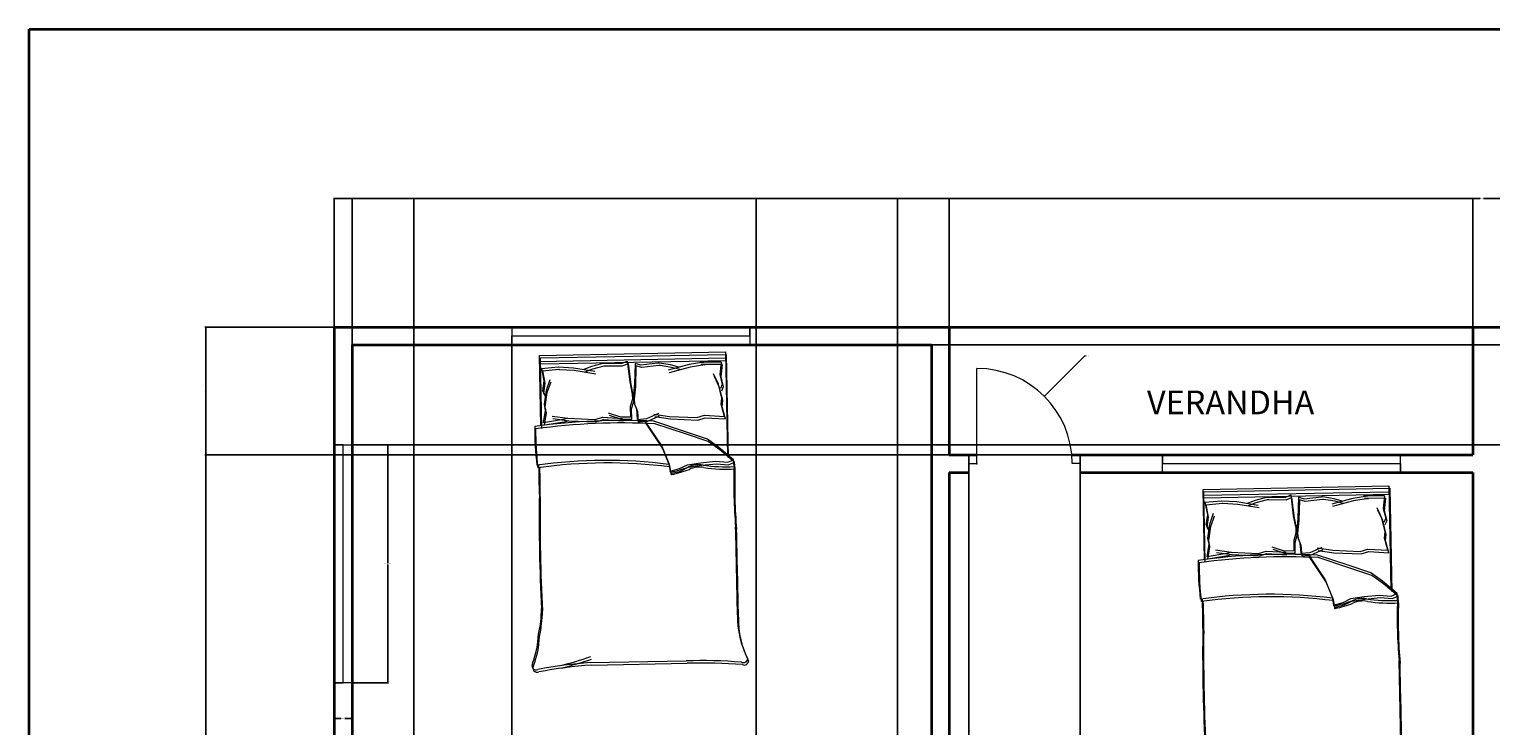
# Model space of a CAD drawing. Units: inches. Extents: x 1721 to 2510, y 1544 to 2360.
# Tile 8 of 10: x 1721 to 2090, y 2185 to 2360. Entities that reach past the tile are written whole.
import ezdxf

# ---------------------------------------------------------------- set-up
doc = ezdxf.new("R2010")
doc.units = ezdxf.units.IN
for name, color, linetype, lineweight in [('A-ANNO-DIMS', 2, 'Continuous', 18), ('A-ANNO-TTLB', 7, 'Continuous', 35), ('A-AREA-IDEN', 7, 'Continuous', 18), ('A-DOOR', 3, 'Continuous', 18), ('A-FURN', 8, 'Continuous', 13), ('A-GLAZ', 4, 'Continuous', 18), ('A-WALL', 7, 'Continuous', 35)]:
    doc.layers.add(name, color=color, linetype=linetype, lineweight=lineweight)
doc.styles.get("Standard").update_dxf_attribs({"font": 'arial.ttf'})
doc.dimstyles.get("Standard").update_dxf_attribs({"dimtxt": 0.18, "dimasz": 0.18, "dimexe": 0.18, "dimexo": 0.0625, "dimgap": 0.09, "dimtad": 0, "dimtih": 1, "dimtoh": 1, "dimdec": 4, "dimzin": 0, "dimdsep": 46, "dimtxsty": 'Standard', "dimcen": 0.09, "dimadec": 0, "dimazin": 0, "dimtfac": 1, "dimtdec": 4, "dimtofl": 0, "dimtmove": 0, "dimatfit": 3, "dimfxl": 1, "dimtolj": 1, "dimtzin": 0, "dimarcsym": 0})

# ---------------------------------------------------------------- blocks, each defined once
blk = doc.blocks.new('BED-DOUBLE')
for p, q in [((39.64, 78.43), (15.52, 78.72)), ((39.64, 78.43), (15.52, 78.72)), ((39.86, 77.8), (15.74, 78.09)), ((39.86, 77.8), (15.74, 78.09)), ((1.93, 30.11), (1.99, 28.4, 3.79)), ((1.93, 30.11), (1.99, 28.4, 3.79)), ((2.15, 29.48), (2.21, 27.77, 3.79)), ((2.15, 29.48), (2.21, 27.77, 3.79)), ((15.66, 30.21), (13.68, 29.32)), ((15.66, 30.21), (13.68, 29.32)), ((15.88, 29.58), (13.89, 28.69)), ((15.88, 29.58), (13.89, 28.69)), ((18.1, 30.79), (15.66, 30.21)), ((18.1, 30.79), (15.66, 30.21)), ((18.31, 30.16), (15.88, 29.58)), ((18.31, 30.16), (15.88, 29.58)), ((18.38, 28.81), (18.1, 30.79)), ((18.38, 28.81), (18.1, 30.79)), ((18.59, 28.18), (18.31, 30.16)), ((18.59, 28.18), (18.31, 30.16)), ((3.5, 28.99), (1.99, 28.4)), ((3.5, 28.99), (1.99, 28.4)), ((1.99, 28.4), (5.58, 25.17)), ((1.99, 28.4), (5.58, 25.17)), ((3.72, 28.36), (2.21, 27.77)), ((3.72, 28.36), (2.21, 27.77)), ((2.21, 27.77), (5.8, 24.54)), ((2.21, 27.77), (5.8, 24.54)), ((3.23, 1.19), (3.55, 27.27)), ((3.23, 1.19), (3.55, 27.27)), ((3.45, 0.56), (3.76, 26.64)), ((3.45, 0.56), (3.76, 26.64)), ((6.54, 28.65), (3.5, 28.99)), ((6.54, 28.65), (3.5, 28.99)), ((6.75, 28.02), (3.72, 28.36)), ((6.75, 28.02), (3.72, 28.36)), ((10.33, 28.91), (6.54, 28.65)), ((10.33, 28.91), (6.54, 28.65)), ((10.55, 28.28), (6.75, 28.02)), ((10.55, 28.28), (6.75, 28.02)), ((13.68, 29.32), (10.33, 28.91)), ((13.68, 29.32), (10.33, 28.91)), ((13.89, 28.69), (10.55, 28.28)), ((13.89, 28.69), (10.55, 28.28)), ((20, 24.39), (18.38, 28.81)), ((20, 24.39), (18.38, 28.81)), ((20.21, 23.76), (18.59, 28.18)), ((20.21, 23.76), (18.59, 28.18)), ((5.58, 25.17), (8.44, 23.01)), ((5.58, 25.17), (8.44, 23.01)), ((5.8, 24.54), (8.66, 22.38)), ((5.8, 24.54), (8.66, 22.38)), ((8.44, 23.01), (13.88, 20.98)), ((8.44, 23.01), (13.88, 20.98)), ((8.66, 22.38), (14.1, 20.35)), ((8.66, 22.38), (14.1, 20.35)), ((24.03, 17.98), (20, 24.39)), ((24.03, 17.98), (20, 24.39)), ((24.24, 17.35), (20.21, 23.76)), ((24.24, 17.35), (20.21, 23.76)), ((13.88, 20.98), (22.02, 18)), ((13.88, 20.98), (22.02, 18)), ((14.1, 20.35), (22.24, 17.37)), ((14.1, 20.35), (22.24, 17.37)), ((9.01, 16.97), (3.98, 17.42)), ((3.98, 17.42), (4.71, 14.34)), ((9.01, 16.97), (3.98, 17.42)), ((3.98, 17.42), (4.71, 14.34)), ((9.23, 16.34), (4.2, 16.8)), ((4.2, 16.8), (4.92, 13.71)), ((9.23, 16.34), (4.2, 16.8)), ((4.2, 16.8), (4.92, 13.71)), ((10.94, 17.49), (9.01, 16.97)), ((10.94, 17.49), (9.01, 16.97)), ((11.15, 16.86), (9.23, 16.34)), ((11.15, 16.86), (9.23, 16.34)), ((17.8, 16.99), (10.94, 17.49)), ((17.8, 16.99), (10.94, 17.49)), ((18.02, 16.36), (11.15, 16.86)), ((18.02, 16.36), (11.15, 16.86)), ((21.75, 16.29), (17.8, 16.99)), ((21.75, 16.29), (17.8, 16.99)), ((21.96, 15.66), (18.02, 16.36)), ((21.96, 15.66), (18.02, 16.36)), ((23.54, 17.35), (20.51, 16.13)), ((23.54, 17.35), (20.51, 16.13)), ((23.75, 16.73), (20.73, 15.5)), ((23.75, 16.73), (20.73, 15.5)), ((25.94, 17.48), (23.54, 17.35)), ((25.94, 17.48), (23.54, 17.35)), ((26.16, 16.85), (23.75, 16.73)), ((26.16, 16.85), (23.75, 16.73)), ((26.07, 14.85), (25.94, 17.48)), ((26.07, 14.85), (25.94, 17.48)), ((26.73, 13.04), (26.07, 14.85)), ((26.73, 13.04), (26.07, 14.85)), ((26.29, 14.22), (26.16, 16.85)), ((26.29, 14.22), (26.16, 16.85)), ((27.61, 14.21), (27.64, 16.84)), ((27.61, 14.21), (27.64, 16.84)), ((27.64, 16.84), (30.05, 16.81)), ((27.64, 16.84), (30.05, 16.81)), ((27.82, 13.58), (27.85, 16.21)), ((27.82, 13.58), (27.85, 16.21)), ((27.85, 16.21), (30.26, 16.18)), ((27.85, 16.21), (30.26, 16.18)), ((34.67, 16.66), (29.65, 17.12)), ((34.67, 16.66), (29.65, 17.12)), ((34.89, 16.03), (29.86, 16.49)), ((34.89, 16.03), (29.86, 16.49)), ((30.05, 16.81), (33.11, 15.7)), ((30.05, 16.81), (33.11, 15.7)), ((30.26, 16.18), (33.33, 15.07)), ((30.26, 16.18), (33.33, 15.07)), ((36.6, 17.19), (34.67, 16.66)), ((36.6, 17.19), (34.67, 16.66)), ((36.81, 16.56), (34.89, 16.03)), ((36.81, 16.56), (34.89, 16.03)), ((43.46, 16.68), (36.6, 17.19)), ((43.46, 16.68), (36.6, 17.19)), ((43.68, 16.05), (36.81, 16.56)), ((43.68, 16.05), (36.81, 16.56)), ((43.46, 16.68), (44.58, 16.98)), ((43.46, 16.68), (44.58, 16.98)), ((47.41, 15.98), (43.46, 16.68)), ((47.41, 15.98), (43.46, 16.68)), ((43.68, 16.05), (44.79, 16.35)), ((43.68, 16.05), (44.79, 16.35)), ((47.62, 15.35), (43.68, 16.05)), ((47.62, 15.35), (43.68, 16.05)), ((44.58, 16.98), (49.58, 17.63)), ((44.58, 16.98), (49.58, 17.63)), ((44.79, 16.35), (49.8, 17)), ((44.79, 16.35), (49.8, 17)), ((49.58, 17.63), (48.98, 14.52)), ((49.58, 17.63), (48.98, 14.52)), ((49.8, 17), (49.19, 13.89)), ((49.8, 17), (49.19, 13.89)), ((50.28, 18.38), (50.07, 0.63)), ((50.28, 18.38), (50.07, 0.63)), ((50.5, 17.75), (50.29, 0)), ((50.5, 17.75), (50.29, 0)), ((4.71, 14.34), (4.5, 12.77)), ((4.71, 14.34), (4.5, 12.77)), ((4.5, 12.77), (5.25, 9.26)), ((4.5, 12.77), (5.25, 9.26)), ((4.92, 13.71), (4.72, 12.14)), ((4.92, 13.71), (4.72, 12.14)), ((4.72, 12.14), (5.46, 8.63)), ((4.72, 12.14), (5.46, 8.63)), ((26.95, 12.41), (26.29, 14.22)), ((26.95, 12.41), (26.29, 14.22)), ((26.39, 8.62), (26.8, 11.77)), ((26.39, 8.62), (26.8, 11.77)), ((26.61, 7.99), (27.01, 11.14)), ((26.61, 7.99), (27.01, 11.14)), ((26.8, 11.77), (26.73, 13.04)), ((26.8, 11.77), (26.73, 13.04)), ((27.01, 11.14), (26.95, 12.41)), ((27.01, 11.14), (26.95, 12.41)), ((27, 11.1), (27.02, 12.38)), ((27, 11.1), (27.02, 12.38)), ((27.53, 7.98), (27, 11.1)), ((27.53, 7.98), (27, 11.1)), ((27.02, 12.38), (27.61, 14.21)), ((27.02, 12.38), (27.61, 14.21)), ((27.22, 10.47), (27.23, 11.75)), ((27.22, 10.47), (27.23, 11.75)), ((27.23, 11.75), (27.82, 13.58)), ((27.23, 11.75), (27.82, 13.58)), ((49.24, 12.96), (48.63, 9.42)), ((49.24, 12.96), (48.63, 9.42)), ((49.46, 12.33), (48.85, 8.79)), ((49.46, 12.33), (48.85, 8.79)), ((48.98, 14.52), (49.24, 12.96)), ((48.98, 14.52), (49.24, 12.96)), ((49.19, 13.89), (49.46, 12.33)), ((49.19, 13.89), (49.46, 12.33)), ((4.25, 9.35), (4.77, 10.37)), ((4.25, 9.35), (4.77, 10.37)), ((4.8, 6.82), (4.25, 9.35)), ((4.8, 6.82), (4.25, 9.35)), ((4.47, 8.72), (4.98, 9.74)), ((4.47, 8.72), (4.98, 9.74)), ((5.02, 6.19), (4.47, 8.72)), ((5.02, 6.19), (4.47, 8.72)), ((5.25, 9.26), (6.37, 6.62)), ((5.25, 9.26), (6.37, 6.62)), ((5.46, 8.63), (6.59, 5.99)), ((5.46, 8.63), (6.59, 5.99)), ((26.09, 3.36), (26.39, 8.62)), ((26.09, 3.36), (26.39, 8.62)), ((26.3, 2.73), (26.61, 7.99)), ((26.3, 2.73), (26.61, 7.99)), ((27.75, 7.35), (27.22, 10.47)), ((27.75, 7.35), (27.22, 10.47)), ((28.04, 2.73), (27.53, 7.98)), ((28.04, 2.73), (27.53, 7.98)), ((48.63, 9.42), (47.61, 6.74)), ((48.63, 9.42), (47.61, 6.74)), ((48.85, 8.79), (47.82, 6.11)), ((48.85, 8.79), (47.82, 6.11)), ((49.63, 9.55), (49.07, 10.55)), ((49.63, 9.55), (49.07, 10.55)), ((49.17, 7.01), (49.63, 9.55)), ((49.17, 7.01), (49.63, 9.55)), ((49.84, 8.92), (49.29, 9.92)), ((49.84, 8.92), (49.29, 9.92)), ((49.39, 6.38), (49.84, 8.92)), ((49.39, 6.38), (49.84, 8.92)), ((4.39, 3.68), (4.8, 6.82)), ((4.39, 3.68), (4.8, 6.82)), ((4.61, 3.05), (5.02, 6.19)), ((4.61, 3.05), (5.02, 6.19)), ((8.71, 3.62), (12.44, 4.09)), ((8.71, 3.62), (12.44, 4.09)), ((12.44, 4.09), (17.76, 5.35)), ((12.44, 4.09), (17.76, 5.35)), ((12.65, 3.46), (17.98, 4.72)), ((12.65, 3.46), (17.98, 4.72)), ((15.1, 4.65), (17.12, 4.04)), ((15.1, 4.65), (17.12, 4.04)), ((15.32, 4.02), (17.34, 3.41)), ((15.32, 4.02), (17.34, 3.41)), ((17.12, 4.04), (19.98, 3.48)), ((17.12, 4.04), (19.98, 3.48)), ((20.3, 3.49), (24.64, 3.85)), ((20.3, 3.49), (24.64, 3.85)), ((24.64, 3.85), (26.09, 3.36)), ((24.64, 3.85), (26.09, 3.36)), ((28.25, 2.1), (27.75, 7.35)), ((28.25, 2.1), (27.75, 7.35)), ((36.97, 3.75), (34.13, 3.08)), ((36.97, 3.75), (34.13, 3.08)), ((41.65, 3.98), (36.28, 5.04)), ((41.65, 3.98), (36.28, 5.04)), ((41.87, 3.35), (36.49, 4.41)), ((41.87, 3.35), (36.49, 4.41)), ((38.96, 4.44), (36.97, 3.75)), ((38.96, 4.44), (36.97, 3.75)), ((39.18, 3.81), (37.19, 3.12)), ((39.18, 3.81), (37.19, 3.12)), ((45.39, 3.65), (41.65, 3.98)), ((45.39, 3.65), (41.65, 3.98)), ((49.7, 3.91), (45.5, 3.63)), ((49.7, 3.91), (45.5, 3.63)), ((49.7, 3.88), (49.17, 7.01)), ((49.7, 3.88), (49.17, 7.01)), ((49.92, 3.25), (49.39, 6.38)), ((49.92, 3.25), (49.39, 6.38)), ((50.07, 0.63), (3.23, 1.19)), ((50.07, 0.63), (3.23, 1.19)), ((50.09, 2.13), (3.25, 2.69)), ((50.09, 2.13), (3.25, 2.69)), ((50.29, 0), (3.45, 0.56)), ((50.29, 0), (3.45, 0.56)), ((50.31, 1.5), (3.47, 2.06)), ((50.31, 1.5), (3.47, 2.06)), ((4.39, 3.68), (9.69, 3.52)), ((4.39, 3.68), (9.69, 3.52)), ((4.61, 3.05), (9.9, 2.89)), ((4.61, 3.05), (9.9, 2.89)), ((9.69, 3.52), (8.71, 3.62)), ((9.69, 3.52), (8.71, 3.62)), ((8.92, 2.99), (12.65, 3.46)), ((8.92, 2.99), (12.65, 3.46)), ((9.9, 2.89), (8.92, 2.99)), ((9.9, 2.89), (8.92, 2.99)), ((17.34, 3.41), (20.2, 2.85)), ((17.34, 3.41), (20.2, 2.85)), ((19.98, 3.48), (20.3, 3.49)), ((19.98, 3.48), (20.3, 3.49)), ((20.2, 2.85), (20.52, 2.86)), ((20.2, 2.85), (20.52, 2.86)), ((20.52, 2.86), (24.86, 3.22)), ((20.52, 2.86), (24.86, 3.22)), ((24.86, 3.22), (26.3, 2.73)), ((24.86, 3.22), (26.3, 2.73)), ((29.46, 3.28), (28.04, 2.73)), ((29.46, 3.28), (28.04, 2.73)), ((29.68, 2.65), (28.25, 2.1)), ((29.68, 2.65), (28.25, 2.1)), ((33.81, 3.08), (29.46, 3.28)), ((33.81, 3.08), (29.46, 3.28)), ((34.03, 2.45), (29.68, 2.65)), ((34.03, 2.45), (29.68, 2.65)), ((34.13, 3.08), (33.81, 3.08)), ((34.13, 3.08), (33.81, 3.08)), ((34.35, 2.45), (34.03, 2.45)), ((34.35, 2.45), (34.03, 2.45)), ((37.19, 3.12), (34.35, 2.45)), ((37.19, 3.12), (34.35, 2.45)), ((45.61, 3.02), (41.87, 3.35)), ((45.61, 3.02), (41.87, 3.35)), ((45.5, 3.63), (45.39, 3.65)), ((45.5, 3.63), (45.39, 3.65)), ((45.71, 3), (45.61, 3.02)), ((45.71, 3), (45.61, 3.02)), ((49.91, 3.28), (45.71, 3)), ((49.91, 3.28), (45.71, 3))]:
    blk.add_line(p, q)
for centre, radius, start, end in [((1.08, 78.52), 1.08, 61.9736, 175.3348), ((1.08, 78.52), 1.08, 61.9736, 175.3348), ((-20.36, 68.78), 22.61, 356.7862, 25.7829), ((-20.36, 68.78), 22.61, 356.7862, 25.7829), ((1.29, 77.89), 1.08, 61.9736, 175.3348), ((1.29, 77.89), 1.08, 61.9736, 175.3348), ((-20.14, 68.15), 22.61, 356.7862, 25.7829), ((-20.14, 68.15), 22.61, 356.7862, 25.7829), ((15.63, 209.12), 130.4, 263.8146, 269.9499), ((15.63, 209.12), 130.4, 263.8146, 269.9499), ((15.85, 208.49), 130.4, 263.8146, 269.9499), ((15.85, 208.49), 130.4, 263.8146, 269.9499), ((70.08, -22.85), 104.34, 102.698, 107.0202), ((70.08, -22.85), 104.34, 102.698, 107.0202), ((34.83, 197.67), 119.34, 272.3106, 278.7239), ((34.83, 197.67), 119.34, 272.3106, 278.7239), ((70.29, -23.48), 104.34, 102.698, 107.0202), ((70.29, -23.48), 104.34, 102.698, 107.0202), ((35.05, 197.04), 119.34, 272.3106, 278.7239), ((35.05, 197.04), 119.34, 272.3106, 278.7239), ((75.53, 69.21), 23.09, 157.2899, 175.9668), ((75.53, 69.21), 23.09, 157.2899, 175.9668), ((75.75, 68.58), 23.09, 157.2899, 175.9668), ((75.75, 68.58), 23.09, 157.2899, 175.9668), ((53.35, 78.73), 1.07, 325.4884, 112.793), ((53.35, 78.73), 1.07, 325.4884, 112.793), ((53.56, 78.1), 1.07, 325.4884, 112.793), ((53.56, 78.1), 1.07, 325.4884, 112.793), ((80.6, 63.5), 29.05, 165.3797, 178.2261), ((80.6, 63.5), 29.05, 165.3797, 178.2261), ((80.81, 62.87), 29.05, 165.3797, 178.2261), ((80.81, 62.87), 29.05, 165.3797, 178.2261), ((4473.12, 14.21), 4471.22, 179.317, 179.60172), ((4473.12, 14.21), 4471.22, 179.317, 179.60172), ((4473.34, 13.58), 4471.22, 179.317, 179.60172), ((4473.34, 13.58), 4471.22, 179.317, 179.60172), ((-421.08, 55.88), 472.73, 357.5425, 1.0334), ((-421.08, 55.88), 472.73, 357.5425, 1.0334), ((-420.87, 55.25), 472.73, 357.5425, 1.0334), ((-420.87, 55.25), 472.73, 357.5425, 1.0334), ((-124.73, 38.32), 126.93, 356.294, 3.1513), ((-124.73, 38.32), 126.93, 356.294, 3.1513), ((-124.51, 37.69), 126.93, 356.294, 3.1513), ((-124.51, 37.69), 126.93, 356.294, 3.1513), ((217.81, 29.18), 166.73, 177.791, 180.323), ((217.81, 29.18), 166.73, 177.791, 180.323), ((218.03, 28.55), 166.73, 177.791, 180.323), ((218.03, 28.55), 166.73, 177.791, 180.323), ((3.1, -5.33), 35.46, 79.1911, 91.8805), ((3.1, -5.33), 35.46, 79.1911, 91.8805), ((3.31, -5.96), 35.46, 79.1911, 91.8805), ((3.31, -5.96), 35.46, 79.1911, 91.8805), ((11.02, 35.47), 6.1, 257.9756, 293.0532), ((11.02, 35.47), 6.1, 257.9756, 293.0532), ((22.96, 2.41), 29.06, 99.9765, 109.1954), ((22.96, 2.41), 29.06, 99.9765, 109.1954), ((23.18, 1.78), 29.06, 99.9765, 109.1954), ((23.18, 1.78), 29.06, 99.9765, 109.1954), ((17.93, 30.85), 0.181, 339.5612, 90.4525), ((17.93, 30.85), 0.181, 339.5612, 90.4525), ((18.15, 30.22), 0.181, 339.5612, 90.4525), ((18.15, 30.22), 0.181, 339.5612, 90.4525), ((11.23, 34.84), 6.1, 257.9756, 293.0532), ((11.23, 34.84), 6.1, 257.9756, 293.0532), ((37.91, 154), 126.46, 261.0993, 276.2154), ((37.91, 154), 126.46, 261.0993, 276.2154), ((38.12, 153.37), 126.46, 261.0993, 276.2154), ((38.12, 153.37), 126.46, 261.0993, 276.2154), ((-29.75, 21.28), 81.65, 358.0366, 4.9188), ((-29.75, 21.28), 81.65, 358.0366, 4.9188), ((-29.53, 20.65), 81.65, 358.0366, 4.9188), ((-29.53, 20.65), 81.65, 358.0366, 4.9188), ((34.68, 179.26), 161.69, 265.4014, 276.097), ((34.68, 179.26), 161.69, 265.4014, 276.097), ((34.89, 178.63), 161.69, 265.4014, 276.097), ((34.89, 178.63), 161.69, 265.4014, 276.097)]:
    blk.add_arc(centre, radius, start, end)
blk = doc.blocks.new('WIN-60IN-A')
for p, q in [((4.5, 60), (0, 60)), ((2.25, 0), (2.25, 60)), ((2.25, 60), (4.5, 60)), ((4.5, 0), (0, 0)), ((0, 0), (2.25, 0))]:
    blk.add_line(p, q)
blk = doc.blocks.new('WIN-60IN-B')
for p, q in [((2.25, 60), (0, 60)), ((0, 60), (4.5, 60)), ((2.25, 0), (2.25, 60)), ((4.5, 0), (0, 0)), ((0, 0), (2.25, 0))]:
    blk.add_line(p, q)
blk = doc.blocks.new('*D20')
at = {"layer": 'A-ANNO-DIMS', "color": 0, "lineweight": -2, "transparency": 16777216}
for p, q in [((1802.56, 2255.45), (1811.68, 2255.45)), ((1811.5, 2255.27), (1811.5, 2225.63)), ((1811.5, 2195.63), (1811.5, 2225.26)), ((1802.56, 2195.45), (1811.68, 2195.45))]:
    blk.add_line(p, q, dxfattribs=at)
at = {"layer": 'A-ANNO-DIMS', "color": 0, "transparency": 16777216}
for points in [[(1811.47, 2255.27), (1811.53, 2255.27), (1811.5, 2255.45)], [(1811.47, 2195.63), (1811.53, 2195.63), (1811.5, 2195.45)]]:
    blk.add_solid(points, dxfattribs=at)
at = {"layer": 'Defpoints', "color": 0, "transparency": 16777216}
for p in [(1802.5, 2255.45), (1811.5, 2255.45), (1802.5, 2195.45)]:
    blk.add_point(p, dxfattribs=at)
at = {"layer": 'A-ANNO-DIMS', "color": 0, "transparency": 16777216, "insert": (1811.5, 2225.45), "char_height": 0.18, "attachment_point": 5}
blk.add_mtext('\\A1;WINDOW B 60 TYP.', dxfattribs=at)
blk = doc.blocks.new('*D21')
at = {"layer": 'A-ANNO-DIMS', "color": 0, "lineweight": -2, "transparency": 16777216}
for p, q in [((1798, 2195.38), (1798, 2186.27)), ((1802.5, 2195.38), (1802.5, 2186.27)), ((1798.18, 2186.45), (1799.79, 2186.45)), ((1802.32, 2186.45), (1800.71, 2186.45))]:
    blk.add_line(p, q, dxfattribs=at)
at = {"layer": 'A-ANNO-DIMS', "color": 0, "transparency": 16777216}
for points in [[(1798.18, 2186.48), (1798.18, 2186.42), (1798, 2186.45)], [(1802.32, 2186.48), (1802.32, 2186.42), (1802.5, 2186.45)]]:
    blk.add_solid(points, dxfattribs=at)
at = {"layer": 'Defpoints', "color": 0, "transparency": 16777216}
for p in [(1798, 2195.45), (1802.5, 2195.45), (1802.5, 2186.45)]:
    blk.add_point(p, dxfattribs=at)
at = {"layer": 'A-ANNO-DIMS', "color": 0, "transparency": 16777216, "insert": (1800.25, 2186.45), "char_height": 0.18, "attachment_point": 5}
blk.add_mtext('\\A1;5 TYP.', dxfattribs=at)
blk = doc.blocks.new('*D40')
at = {"layer": 'A-ANNO-DIMS', "color": 0, "lineweight": -2, "transparency": 16777216}
for p, q in [((1798, 2285.19), (1798, 2317.71)), ((1798.18, 2317.53), (2086.86, 2317.53)), ((2376.32, 2317.53), (2087.65, 2317.53)), ((2376.5, 2285.19), (2376.5, 2317.71))]:
    blk.add_line(p, q, dxfattribs=at)
at = {"layer": 'A-ANNO-DIMS', "color": 0, "transparency": 16777216}
for points in [[(1798.18, 2317.56), (1798.18, 2317.5), (1798, 2317.53)], [(2376.32, 2317.56), (2376.32, 2317.5), (2376.5, 2317.53)]]:
    blk.add_solid(points, dxfattribs=at)
at = {"layer": 'Defpoints', "color": 0, "transparency": 16777216}
for p in [(2376.5, 2317.53), (1798, 2285.13), (2376.5, 2285.13)]:
    blk.add_point(p, dxfattribs=at)
at = {"layer": 'A-ANNO-DIMS', "color": 0, "transparency": 16777216, "insert": (2087.25, 2317.53), "char_height": 0.18, "attachment_point": 5}
blk.add_mtext('\\A1;578.5', dxfattribs=at)
blk = doc.blocks.new('*D41')
at = {"layer": 'A-ANNO-DIMS', "color": 0, "lineweight": -2, "transparency": 16777216}
for p, q in [((1797.94, 2285.13), (1765.42, 2285.13)), ((1765.6, 2284.95), (1765.6, 1987.06)), ((1765.6, 1688.81), (1765.6, 1986.7)), ((1797.94, 1688.63), (1765.42, 1688.63))]:
    blk.add_line(p, q, dxfattribs=at)
at = {"layer": 'A-ANNO-DIMS', "color": 0, "transparency": 16777216}
for points in [[(1765.57, 2284.95), (1765.63, 2284.95), (1765.6, 2285.13)], [(1765.57, 1688.81), (1765.63, 1688.81), (1765.6, 1688.63)]]:
    blk.add_solid(points, dxfattribs=at)
at = {"layer": 'Defpoints', "color": 0, "transparency": 16777216}
for p in [(1765.6, 2285.13), (1798, 2285.13), (1798, 1688.63)]:
    blk.add_point(p, dxfattribs=at)
at = {"layer": 'A-ANNO-DIMS', "color": 0, "transparency": 16777216, "insert": (1765.6, 1986.88), "char_height": 0.18, "attachment_point": 5}
blk.add_mtext('\\A1;596.5', dxfattribs=at)
blk = doc.blocks.new('*D46')
at = {"layer": 'A-ANNO-DIMS', "color": 0, "lineweight": -2, "transparency": 16777216}
for p, q in [((1953, 2285.19), (1953, 2317.71)), ((1953.18, 2317.53), (2018.72, 2317.53)), ((2084.82, 2317.53), (2019.28, 2317.53)), ((2085, 2285.19), (2085, 2317.71))]:
    blk.add_line(p, q, dxfattribs=at)
at = {"layer": 'A-ANNO-DIMS', "color": 0, "transparency": 16777216}
for points in [[(1953.18, 2317.56), (1953.18, 2317.5), (1953, 2317.53)], [(2084.82, 2317.56), (2084.82, 2317.5), (2085, 2317.53)]]:
    blk.add_solid(points, dxfattribs=at)
at = {"layer": 'Defpoints', "color": 0, "transparency": 16777216}
for p in [(2085, 2317.53), (1953, 2285.13), (2085, 2285.13)]:
    blk.add_point(p, dxfattribs=at)
at = {"layer": 'A-ANNO-DIMS', "color": 0, "transparency": 16777216, "insert": (2019, 2317.53), "char_height": 0.18, "attachment_point": 5}
blk.add_mtext('\\A1;132', dxfattribs=at)
blk = doc.blocks.new('*D55')
at = {"layer": 'A-ANNO-DIMS', "color": 0, "lineweight": -2, "transparency": 16777216}
for p, q in [((2084.94, 2285.13), (1765.42, 2285.13)), ((1765.6, 2284.95), (1765.6, 2269.22)), ((1765.6, 2253.12), (1765.6, 2268.85)), ((2084.94, 2252.94), (1765.42, 2252.94))]:
    blk.add_line(p, q, dxfattribs=at)
at = {"layer": 'A-ANNO-DIMS', "color": 0, "transparency": 16777216}
for points in [[(1765.57, 2284.95), (1765.63, 2284.95), (1765.6, 2285.13)], [(1765.57, 2253.12), (1765.63, 2253.12), (1765.6, 2252.94)]]:
    blk.add_solid(points, dxfattribs=at)
at = {"layer": 'Defpoints', "color": 0, "transparency": 16777216}
for p in [(1765.6, 2285.13), (2085, 2285.13), (2085, 2252.94)]:
    blk.add_point(p, dxfattribs=at)
at = {"layer": 'A-ANNO-DIMS', "color": 0, "transparency": 16777216, "insert": (1765.6, 2269.04), "char_height": 0.18, "attachment_point": 5}
blk.add_mtext('\\A1;32.19', dxfattribs=at)
blk = doc.blocks.new('*D56')
at = {"layer": 'A-ANNO-DIMS', "color": 0, "lineweight": -2, "transparency": 16777216}
for p, q in [((1802.5, 2280.57), (1802.5, 1606.75)), ((1842.73, 2280.57), (1842.73, 1606.75)), ((1802.68, 1606.93), (1822.15, 1606.93)), ((1842.55, 1606.93), (1823.08, 1606.93))]:
    blk.add_line(p, q, dxfattribs=at)
at = {"layer": 'A-ANNO-DIMS', "color": 0, "transparency": 16777216}
for points in [[(1802.68, 1606.96), (1802.68, 1606.9), (1802.5, 1606.93)], [(1842.55, 1606.96), (1842.55, 1606.9), (1842.73, 1606.93)]]:
    blk.add_solid(points, dxfattribs=at)
at = {"layer": 'Defpoints', "color": 0, "transparency": 16777216}
for p in [(1802.5, 2280.63), (1842.73, 2280.63), (1842.73, 1606.93)]:
    blk.add_point(p, dxfattribs=at)
at = {"layer": 'A-ANNO-DIMS', "color": 0, "transparency": 16777216, "insert": (1822.61, 1606.93), "char_height": 0.18, "attachment_point": 5}
blk.add_mtext('\\A1;40.224', dxfattribs=at)
blk = doc.blocks.new('*D57')
at = {"layer": 'A-ANNO-DIMS', "color": 0, "lineweight": -2, "transparency": 16777216}
for p, q in [((1802.56, 2280.63), (2409.08, 2280.63)), ((2408.9, 2280.45), (2408.9, 2268.22)), ((2408.9, 2255.63), (2408.9, 2267.86)), ((1802.56, 2255.45), (2409.08, 2255.45))]:
    blk.add_line(p, q, dxfattribs=at)
at = {"layer": 'A-ANNO-DIMS', "color": 0, "transparency": 16777216}
for points in [[(2408.87, 2280.45), (2408.93, 2280.45), (2408.9, 2280.63)], [(2408.87, 2255.63), (2408.93, 2255.63), (2408.9, 2255.45)]]:
    blk.add_solid(points, dxfattribs=at)
at = {"layer": 'Defpoints', "color": 0, "transparency": 16777216}
for p in [(1802.5, 2280.63), (1802.5, 2255.45), (2408.9, 2255.45)]:
    blk.add_point(p, dxfattribs=at)
at = {"layer": 'A-ANNO-DIMS', "color": 0, "transparency": 16777216, "insert": (2408.9, 2268.04), "char_height": 0.18, "attachment_point": 5}
blk.add_mtext('\\A1;25.18', dxfattribs=at)
blk = doc.blocks.new('*D59')
at = {"layer": 'A-ANNO-DIMS', "color": 0, "lineweight": -2, "transparency": 16777216}
for p, q in [((1904.34, 1857.19), (1904.34, 2317.71)), ((1904.52, 2317.53), (1921.76, 2317.53)), ((1939.78, 2317.53), (1922.54, 2317.53)), ((1939.96, 1857.19), (1939.96, 2317.71))]:
    blk.add_line(p, q, dxfattribs=at)
at = {"layer": 'A-ANNO-DIMS', "color": 0, "transparency": 16777216}
for points in [[(1904.52, 2317.56), (1904.52, 2317.5), (1904.34, 2317.53)], [(1939.78, 2317.56), (1939.78, 2317.5), (1939.96, 2317.53)]]:
    blk.add_solid(points, dxfattribs=at)
at = {"layer": 'Defpoints', "color": 0, "transparency": 16777216}
for p in [(1939.96, 2317.53), (1904.34, 1857.13), (1939.96, 1857.13)]:
    blk.add_point(p, dxfattribs=at)
at = {"layer": 'A-ANNO-DIMS', "color": 0, "transparency": 16777216, "insert": (1922.15, 2317.53), "char_height": 0.18, "attachment_point": 5}
blk.add_mtext('\\A1;35.62', dxfattribs=at)
blk = doc.blocks.new('*D62')
at = {"layer": 'A-ANNO-DIMS', "color": 0, "lineweight": -2, "transparency": 16777216}
for p, q in [((1957.99, 2252.88), (1957.99, 1606.75)), ((1986.02, 2252.88), (1986.02, 1606.75)), ((1958.17, 1606.93), (1971.61, 1606.93)), ((1985.84, 1606.93), (1972.4, 1606.93))]:
    blk.add_line(p, q, dxfattribs=at)
at = {"layer": 'A-ANNO-DIMS', "color": 0, "transparency": 16777216}
for points in [[(1958.17, 1606.96), (1958.17, 1606.9), (1957.99, 1606.93)], [(1985.84, 1606.96), (1985.84, 1606.9), (1986.02, 1606.93)]]:
    blk.add_solid(points, dxfattribs=at)
at = {"layer": 'Defpoints', "color": 0, "transparency": 16777216}
for p in [(1957.99, 2252.94), (1986.02, 2252.94), (1986.02, 1606.93)]:
    blk.add_point(p, dxfattribs=at)
at = {"layer": 'A-ANNO-DIMS', "color": 0, "transparency": 16777216, "insert": (1972.01, 1606.93), "char_height": 0.18, "attachment_point": 5}
blk.add_mtext('\\A1;28.03', dxfattribs=at)
blk = doc.blocks.new('*D66')
at = {"layer": 'A-ANNO-DIMS', "color": 0, "lineweight": -2, "transparency": 16777216}
for p, q in [((1802.5, 2051.19), (1802.5, 2317.71)), ((1802.68, 2317.53), (1809.89, 2317.53)), ((1817.87, 2317.53), (1810.66, 2317.53)), ((1818.05, 2051.19), (1818.05, 2317.71))]:
    blk.add_line(p, q, dxfattribs=at)
at = {"layer": 'A-ANNO-DIMS', "color": 0, "transparency": 16777216}
for points in [[(1802.68, 2317.56), (1802.68, 2317.5), (1802.5, 2317.53)], [(1817.87, 2317.56), (1817.87, 2317.5), (1818.05, 2317.53)]]:
    blk.add_solid(points, dxfattribs=at)
at = {"layer": 'Defpoints', "color": 0, "transparency": 16777216}
for p in [(1818.05, 2317.53), (1802.5, 2051.13), (1818.05, 2051.13)]:
    blk.add_point(p, dxfattribs=at)
at = {"layer": 'A-ANNO-DIMS', "color": 0, "transparency": 16777216, "insert": (1810.28, 2317.53), "char_height": 0.18, "attachment_point": 5}
blk.add_mtext('\\A1;15.55', dxfattribs=at)
blk = doc.blocks.new('*D85')
at = {"layer": 'A-ANNO-DIMS', "color": 0, "lineweight": -2, "transparency": 16777216}
for p, q in [((1987.16, 2277.87), (1977.1, 2267.79)), ((1987.34, 2277.87), (1987.16, 2277.87)), ((1959.9, 2250.66), (1960.08, 2250.66)), ((1959.99, 2250.57), (1959.99, 2250.75))]:
    blk.add_line(p, q, dxfattribs=at)
at = {"layer": 'A-ANNO-DIMS', "color": 0, "transparency": 16777216}
blk.add_solid([(1977.08, 2267.81), (1977.12, 2267.77), (1976.97, 2267.66)], dxfattribs=at)
at = {"layer": 'Defpoints', "color": 0, "transparency": 16777216}
for p in [(1976.97, 2267.66), (1959.99, 2250.66)]:
    blk.add_point(p, dxfattribs=at)
at = {"layer": 'A-ANNO-DIMS', "color": 0, "transparency": 16777216, "insert": (1987.82, 2277.87), "char_height": 0.18, "attachment_point": 5}
blk.add_mtext('\\A1;R24.03', dxfattribs=at)

msp = doc.modelspace()

# ---------------------------------------------------------------- linework, layer by layer
at = {"layer": 'A-ANNO-TTLB'}
msp.add_lwpolyline([(1721.1268, 2360.2177), (2509.707, 2360.2177), (2509.707, 1544.3037), (1721.1268, 1544.3037)], close=True, dxfattribs=at)
at = {"layer": 'A-DOOR'}
for p, q in [((1959.9903, 2250.6915), (1959.9903, 2274.6915)), ((1957.9903, 2252.9415), (1957.9903, 2248.4415)), ((1986.0213, 2252.9415), (1986.0213, 2248.4415)), ((1957.9903, 2248.4415), (1957.9903, 2250.6915)), ((1957.9903, 2250.6915), (1959.9903, 2250.6915)), ((1986.0213, 2250.6915), (1984.0213, 2250.6915)), ((1986.0213, 2248.4415), (1986.0213, 2250.6915))]:
    msp.add_line(p, q, dxfattribs=at)
msp.add_arc((1959.9903, 2250.6605), 24.031, 0.073943, 90, dxfattribs=at)
at = {"layer": 'A-WALL'}
for p, q in [((1798.0024, 2285.1298), (1953.0024, 2285.1298)), ((1798.0024, 2285.1298), (1798.0024, 1688.6298)), ((1953.0024, 2285.1298), (1953.0024, 2252.9415)), ((1953.0024, 2285.1298), (2221.5024, 2285.1298)), ((2085.0024, 2285.1298), (2085.0024, 2252.9415)), ((2085.0024, 2285.1298), (2089.5024, 2285.1298)), ((1802.5024, 2280.6298), (1948.5024, 2280.6298)), ((1802.5024, 2280.6298), (1802.5024, 2148.6298)), ((1948.5024, 2280.6298), (1948.5024, 2148.6298)), ((1953.0024, 2252.9415), (1959.9903, 2252.9415)), ((1983.9128, 2252.9415), (2085.0024, 2252.9415)), ((1953.0024, 2248.4415), (1957.9903, 2248.4415)), ((1953.0024, 2248.4415), (1953.0024, 2120.9415)), ((1986.0213, 2248.4415), (2085.0024, 2248.4415)), ((2085.0024, 2248.4415), (2085.0024, 2120.9415))]:
    msp.add_line(p, q, dxfattribs=at)

# ---------------------------------------------------------------- block references
at = {"layer": 'A-FURN'}
for p, rotation in [((1900.0175, 2279.5069), 181.7686830003587), ((2067.2396, 2245.759), 181.7686830003585)]:
    msp.add_blockref('BED-DOUBLE', p, dxfattribs=dict(at, rotation=rotation))
at = {"layer": 'A-GLAZ', "extrusion": (0, 0, -1), "zscale": -1, "rotation": 90}
msp.add_blockref('WIN-60IN-A', (-1842.7268, 2280.6294), dxfattribs=at)
at = {"layer": 'A-GLAZ'}
msp.add_blockref('WIN-60IN-B', (1798.002, 2195.447), dxfattribs=at)
at = {"layer": 'A-GLAZ', "rotation": 270}
msp.add_blockref('WIN-60IN-A', (2006.775, 2252.942), dxfattribs=at)

# ---------------------------------------------------------------- texts
at = {"layer": 'A-AREA-IDEN', "insert": (2002.8438, 2269.1281), "char_height": 6, "attachment_point": 1}
msp.add_mtext_dynamic_manual_height_columns('VERANDHA', width=124.715263, gutter_width=12.5, heights=[0], dxfattribs=at)

# ---------------------------------------------------------------- dimensions: what is measured, and where the dimension line sits
at = {"layer": 'A-ANNO-DIMS'}
for base, p1, p2, override, picture, middle in [((2376.5024, 2317.5298), (1798.0024, 2285.1298), (2376.5024, 2285.1298), {"dimdec": 1, "dimlfac": 1, "dimrnd": 0, "dimzin": 0, "dimdsep": 46, "dimlunit": 2}, '*D40', (2087.2524, 2317.5298)), ((1818.0518, 2317.5298), (1802.5024, 2051.1298), (1818.0518, 2051.1298), {"dimdec": 2, "dimlfac": 1, "dimrnd": 0, "dimzin": 0, "dimdsep": 46, "dimlunit": 2}, '*D66', (1810.2771, 2317.5298)), ((1939.9594, 2317.5298), (1904.3387, 1857.1298), (1939.9594, 1857.1298), {"dimdec": 2, "dimlfac": 1, "dimrnd": 0, "dimzin": 0, "dimdsep": 46, "dimlunit": 2}, '*D59', (1922.149, 2317.5298)), ((2085.0024, 2317.5298), (1953.0024, 2285.1298), (2085.0024, 2285.1298), {"dimdec": 0, "dimlfac": 1, "dimrnd": 0, "dimzin": 0, "dimdsep": 46, "dimlunit": 2}, '*D46', (2019.0024, 2317.5298)), ((1842.7265, 1606.9297), (1802.5024, 2280.6298), (1842.7265, 2280.6298), {"dimdec": 3, "dimlfac": 1, "dimrnd": 0, "dimzin": 0, "dimdsep": 46, "dimlunit": 2}, '*D56', (1822.6145, 1606.9297)), ((1986.0213, 1606.9297), (1957.9903, 2252.9415), (1986.0213, 2252.9415), {"dimdec": 2, "dimlfac": 1, "dimrnd": 0, "dimzin": 0, "dimdsep": 46, "dimlunit": 2}, '*D62', (1972.0058, 1606.9297))]:
    dim = msp.add_linear_dim(base=base, p1=p1, p2=p2, dimstyle='Standard', override=override, dxfattribs=at)
    dim.commit()
    dim.dimension.update_dxf_attribs({"geometry": picture, "text_midpoint": middle})
for base, p1, p2, override, picture, middle in [((1765.6024, 2285.1298), (1798.0024, 1688.6298), (1798.0024, 2285.1298), {"dimdec": 1, "dimlfac": 1, "dimrnd": 0, "dimzin": 0, "dimdsep": 46, "dimlunit": 2}, '*D41', (1765.6024, 1986.8798)), ((1765.6024, 2285.1298), (2085.0024, 2252.9415), (2085.0024, 2285.1298), {"dimdec": 2, "dimlfac": 1, "dimrnd": 0, "dimzin": 0, "dimdsep": 46, "dimlunit": 2}, '*D55', (1765.6024, 2269.0357)), ((2408.9024, 2255.4473), (1802.5024, 2280.6298), (1802.5024, 2255.4473), {"dimdec": 2, "dimlfac": 1, "dimrnd": 0, "dimzin": 0, "dimdsep": 46, "dimlunit": 2}, '*D57', (2408.9024, 2268.0386))]:
    dim = msp.add_linear_dim(base=base, p1=p1, p2=p2, angle=90, dimstyle='Standard', override=override, dxfattribs=at)
    dim.commit()
    dim.dimension.update_dxf_attribs({"geometry": picture, "text_midpoint": middle})
dim = msp.add_radius_dim(center=(1959.9903, 2250.6605), mpoint=(1976.9719, 2267.6639), dimstyle='Standard', override={"dimdec": 2, "dimlfac": 1, "dimrnd": 0, "dimzin": 0, "dimdsep": 46, "dimlunit": 2}, dxfattribs=at)
dim.commit()
dim.dimension.update_dxf_attribs({"geometry": '*D85', "text_midpoint": (1987.8207, 2277.8659), "dimtype": 164})
dim = msp.add_linear_dim(base=(1811.5024, 2255.4473), p1=(1802.5024, 2195.4473), p2=(1802.5024, 2255.4473), angle=90, text='WINDOW B <> TYP.', dimstyle='Standard', override={"dimdec": 0, "dimlfac": 1, "dimrnd": 0, "dimzin": 0, "dimdsep": 46, "dimlunit": 2}, dxfattribs=at)
dim.commit()
dim.dimension.update_dxf_attribs({"geometry": '*D20', "text_midpoint": (1811.5024, 2225.4473)})
dim = msp.add_linear_dim(base=(1802.5024123219, 2186.4473344495), p1=(1798.0024123219, 2195.4473344495), p2=(1802.5024123219, 2195.4473344495), text='<> TYP.', dimstyle='Standard', override={"dimdec": 0, "dimlfac": 1, "dimrnd": 0, "dimzin": 0, "dimdsep": 46, "dimlunit": 2}, dxfattribs=at)
dim.commit()
dim.dimension.update_dxf_attribs({"geometry": '*D21', "text_midpoint": (1800.2524123219, 2186.4473344495)})

doc.saveas('drawing.dxf')
